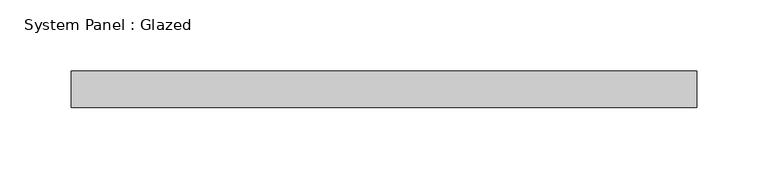
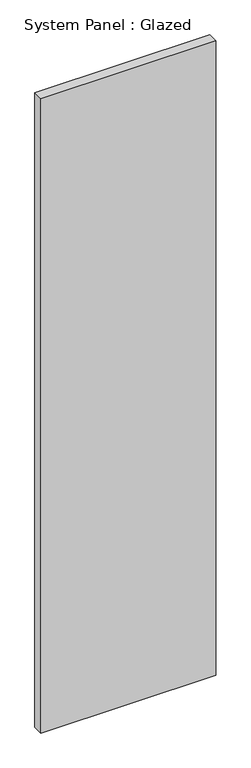
"""IFC4 building model written with IfcOpenShell, lengths in millimetres: plate geometry, System Panel : Glazed."""

from ifc_helpers import new_model, si_unit, origin, origin_with_axes, place, context, project, spatial, polyline, outline, extrude, source, transform, mapped, element, save


def system_panel_glazed_29222c04(model_context):
    return source(origin(), model_context, "Body", "SweptSolid", [
        extrude(outline(polyline([(219.075, 19.05), (-219.075, 19.05), (-219.075, 44.45), (219.075, 44.45), (219.075, 19.05)])), origin_with_axes(), (0.0, 0.0, 1.0), 1678.4265918),
    ])


if __name__ == "__main__":
    model = new_model("IFC4")
    model_context = context("Model", 3, world=origin())
    ifc_project = project(units=[si_unit("LENGTHUNIT", "METRE", prefix="MILLI")], contexts=[model_context])
    site = spatial("IfcSite", under=ifc_project)
    building = spatial("IfcBuilding", under=site)
    placement = place(None, origin())
    system_panel_glazed_shape = system_panel_glazed_29222c04(model_context)
    element("IfcPlate", 1, ObjectType="System Panel : Glazed", at=placement, inside=building, context=model_context, shape_type="MappedRepresentation", body=[
        mapped(system_panel_glazed_shape, transform((0.0, 0.0, 0.0), x_axis=(1.0, 0.0, 0.0), y_axis=(0.0, 1.0, 0.0), z_axis=(0.0, 0.0, 1.0))),
    ])
    save(model, "model.ifc")

# Revit data of these elements
# Type "System Panel : Glazed"
#   Construction Type Id = "GSP4R"
#   Analytic Construction = "1/8 in Pilkington single glazing"
#   Visual Light Transmittance = 0.9
#   Solar Heat Gain Coefficient = 0.86
#   Heat Transfer Coefficient (U) = 1.18115 BTU/(h·ft²·°F)
#   Define Thermal Properties by = 1
# Element 1 (IfcPlate, "System Panel : Glazed")
#   Materials on its faces: "Glass"
# Materials
#   "Glass": class "Glass", colour RGB 0 128 192, transparency 0.75, Description = "Soda Lime Glass", Cost = 0
